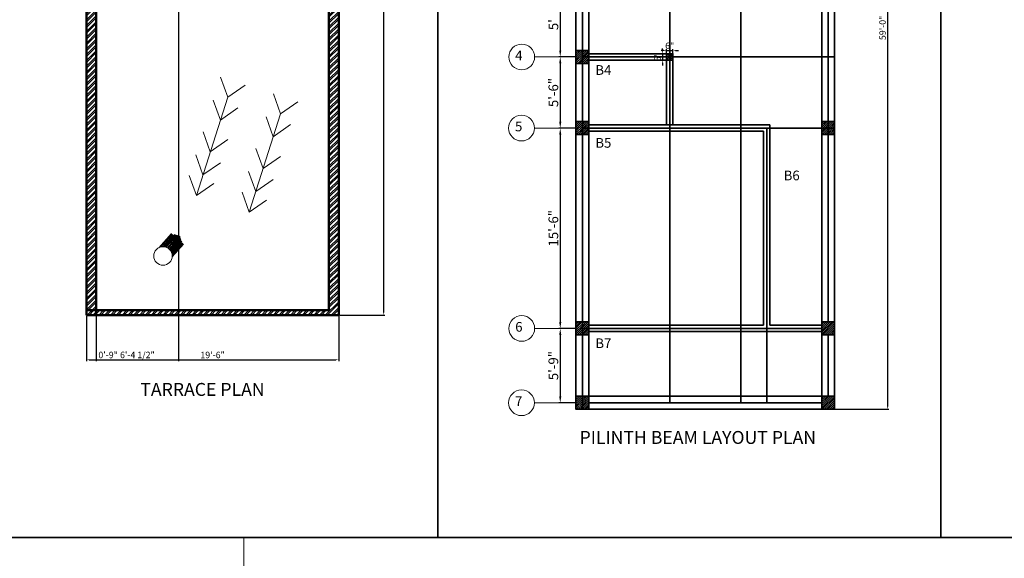
# Model space of a CAD drawing. Units: millimetres. Extents: x 20768 to 23556, y 50760 to 52704.
# Tile 30 of 36: x 21642 to 22556, y 51604 to 52104. Entities that reach past the tile are written whole.
import ezdxf

# ---------------------------------------------------------------- set-up
doc = ezdxf.new("R2010")
doc.units = ezdxf.units.MM
for name, color, linetype, lineweight in [('A-ANNO-SCHD', 7, 'Continuous', 18), ('A-ANNO-TEXT', 7, 'Continuous', 18), ('A-ANNO-TTLB', 7, 'Continuous', 35), ('A-ROOF', 30, 'Continuous', 18), ('A-WALL', 7, 'Continuous', 50), ('A-WALL-PATT', 8, 'Continuous', 13), ('S-ANNO-DIMS', 2, 'Continuous', 18), ('S-ANNO-TEXT', 6, 'Continuous', 18), ('S-BEAM', 3, 'Continuous', 35), ('S-COLS', 20, 'Continuous', 35), ('S-COLS-PATT', 8, 'Continuous', 13), ('S-GRID', 1, 'Continuous', 18)]:
    doc.layers.add(name, color=color, linetype=linetype, lineweight=lineweight)
doc.styles.get("Standard").update_dxf_attribs({"font": 'arial.ttf'})
doc.dimstyles.new('ISO-25', dxfattribs={"dimtxt": 6, "dimasz": 2.5, "dimexe": 1.25, "dimexo": 0.625, "dimtad": 1, "dimdec": 0, "dimlunit": 3, "dimtxsty": 'Standard', "dimcen": 2.5, "dimadec": 0, "dimazin": 0, "dimtfac": 1, "dimtdec": 0, "dimtmove": 0, "dimatfit": 3, "dimfxl": 1, "dimarcsym": 0})
pattern_1 = [(45, (102.9326, 0), (-0.898025612, 0.898025612), [])]

# ---------------------------------------------------------------- blocks, each defined once
blk = doc.blocks.new('*D37')
at = {"layer": 'Defpoints', "color": 0, "transparency": 16777216}
for p in [(22158.2, 52129.51), (22143.63, 52069.51), (22158.2, 52069.51)]:
    blk.add_point(p, dxfattribs=at)
at = {"layer": 'S-ANNO-DIMS', "color": 0, "lineweight": -2, "transparency": 16777216}
for p, q in [((22157.58, 52129.51), (22142.38, 52129.51)), ((22143.63, 52123.51), (22143.63, 52075.51)), ((22157.58, 52069.51), (22142.38, 52069.51))]:
    blk.add_line(p, q, dxfattribs=at)
at = {"layer": 'S-ANNO-DIMS', "color": 0, "transparency": 16777216}
for points in [[(22142.63, 52123.51), (22144.63, 52123.51), (22143.63, 52129.51)], [(22142.63, 52075.51), (22144.63, 52075.51), (22143.63, 52069.51)]]:
    blk.add_solid(points, dxfattribs=at)
at = {"layer": 'S-ANNO-DIMS', "color": 0, "transparency": 16777216, "insert": (22138.43, 52099.51), "char_height": 9, "attachment_point": 5, "rotation": 90}
blk.add_mtext("5'", dxfattribs=at)
blk = doc.blocks.new('*D38')
at = {"layer": 'Defpoints', "color": 0, "transparency": 16777216}
for p in [(22158.2, 52069.51), (22143.63, 52003.51), (22158.2, 52003.51)]:
    blk.add_point(p, dxfattribs=at)
at = {"layer": 'S-ANNO-DIMS', "color": 0, "lineweight": -2, "transparency": 16777216}
for p, q in [((22157.58, 52069.51), (22142.38, 52069.51)), ((22143.63, 52063.51), (22143.63, 52009.51)), ((22157.58, 52003.51), (22142.38, 52003.51))]:
    blk.add_line(p, q, dxfattribs=at)
at = {"layer": 'S-ANNO-DIMS', "color": 0, "transparency": 16777216}
for points in [[(22142.63, 52063.51), (22144.63, 52063.51), (22143.63, 52069.51)], [(22142.63, 52009.51), (22144.63, 52009.51), (22143.63, 52003.51)]]:
    blk.add_solid(points, dxfattribs=at)
at = {"layer": 'S-ANNO-DIMS', "color": 0, "transparency": 16777216, "insert": (22138.41, 52036.51), "char_height": 9, "attachment_point": 5, "rotation": 90}
blk.add_mtext('5\'-6"', dxfattribs=at)
blk = doc.blocks.new('*D39')
at = {"layer": 'Defpoints', "color": 0, "transparency": 16777216}
for p in [(22158.2, 52003.51), (22143.63, 51817.51), (22158.2, 51817.51)]:
    blk.add_point(p, dxfattribs=at)
at = {"layer": 'S-ANNO-DIMS', "color": 0, "lineweight": -2, "transparency": 16777216}
for p, q in [((22157.58, 52003.51), (22142.38, 52003.51)), ((22143.63, 51997.51), (22143.63, 51823.51)), ((22157.58, 51817.51), (22142.38, 51817.51))]:
    blk.add_line(p, q, dxfattribs=at)
at = {"layer": 'S-ANNO-DIMS', "color": 0, "transparency": 16777216}
for points in [[(22142.63, 51997.51), (22144.63, 51997.51), (22143.63, 52003.51)], [(22142.63, 51823.51), (22144.63, 51823.51), (22143.63, 51817.51)]]:
    blk.add_solid(points, dxfattribs=at)
at = {"layer": 'S-ANNO-DIMS', "color": 0, "transparency": 16777216, "insert": (22138.41, 51910.51), "char_height": 9, "attachment_point": 5, "rotation": 90}
blk.add_mtext('15\'-6"', dxfattribs=at)
blk = doc.blocks.new('*D40')
at = {"layer": 'Defpoints', "color": 0, "transparency": 16777216}
for p in [(22158.2, 51817.51), (22143.63, 51748.51), (22158.2, 51748.51)]:
    blk.add_point(p, dxfattribs=at)
at = {"layer": 'S-ANNO-DIMS', "color": 0, "lineweight": -2, "transparency": 16777216}
for p, q in [((22157.58, 51817.51), (22142.38, 51817.51)), ((22143.63, 51811.51), (22143.63, 51754.51)), ((22157.58, 51748.51), (22142.38, 51748.51))]:
    blk.add_line(p, q, dxfattribs=at)
at = {"layer": 'S-ANNO-DIMS', "color": 0, "transparency": 16777216}
for points in [[(22142.63, 51811.51), (22144.63, 51811.51), (22143.63, 51817.51)], [(22142.63, 51754.51), (22144.63, 51754.51), (22143.63, 51748.51)]]:
    blk.add_solid(points, dxfattribs=at)
at = {"layer": 'S-ANNO-DIMS', "color": 0, "transparency": 16777216, "insert": (22138.41, 51783.01), "char_height": 9, "attachment_point": 5, "rotation": 90}
blk.add_mtext('5\'-9"', dxfattribs=at)
blk = doc.blocks.new('*D43')
at = {"layer": 'Defpoints', "color": 0, "transparency": 16777216}
for p in [(22242.2, 52072.51), (22248.2, 52075.41), (22248.2, 52072.51)]:
    blk.add_point(p, dxfattribs=at)
at = {"layer": 'S-ANNO-DIMS', "color": 0, "lineweight": -2, "transparency": 16777216}
for p, q in [((22239.7, 52075.41), (22237.2, 52075.41)), ((22242.2, 52073.13), (22242.2, 52076.66)), ((22242.2, 52075.41), (22248.2, 52075.41)), ((22248.2, 52073.13), (22248.2, 52076.66)), ((22250.7, 52075.41), (22253.2, 52075.41))]:
    blk.add_line(p, q, dxfattribs=at)
at = {"layer": 'S-ANNO-DIMS', "color": 0, "transparency": 16777216}
for points in [[(22239.7, 52075.83), (22239.7, 52075), (22242.2, 52075.41)], [(22250.7, 52075.83), (22250.7, 52075), (22248.2, 52075.41)]]:
    blk.add_solid(points, dxfattribs=at)
at = {"layer": 'S-ANNO-DIMS', "color": 0, "transparency": 16777216, "insert": (22245.2, 52079.1), "char_height": 6, "attachment_point": 5}
blk.add_mtext('6"', dxfattribs=at)
blk = doc.blocks.new('*D44')
at = {"layer": 'Defpoints', "color": 0, "transparency": 16777216}
for p in [(22242.2, 52072.51), (22238.36, 52066.51), (22242.2, 52066.51)]:
    blk.add_point(p, dxfattribs=at)
at = {"layer": 'S-ANNO-DIMS', "color": 0, "lineweight": -2, "transparency": 16777216}
for p, q in [((22238.36, 52075.01), (22238.36, 52077.51)), ((22241.58, 52072.51), (22237.11, 52072.51)), ((22238.36, 52072.51), (22238.36, 52066.51)), ((22241.58, 52066.51), (22237.11, 52066.51)), ((22238.36, 52064.01), (22238.36, 52061.51))]:
    blk.add_line(p, q, dxfattribs=at)
at = {"layer": 'S-ANNO-DIMS', "color": 0, "transparency": 16777216}
for points in [[(22237.95, 52075.01), (22238.78, 52075.01), (22238.36, 52072.51)], [(22237.95, 52064.01), (22238.78, 52064.01), (22238.36, 52066.51)]]:
    blk.add_solid(points, dxfattribs=at)
at = {"layer": 'S-ANNO-DIMS', "color": 0, "transparency": 16777216, "insert": (22234.68, 52069.51), "char_height": 6, "attachment_point": 5, "rotation": 90}
blk.add_mtext('6"', dxfattribs=at)
blk = doc.blocks.new('GRID-BUBBLE')
blk.add_line((47.87, 11.93), (23.87, 11.93))
blk.add_circle((11.93, 11.93), 11.93)
blk = doc.blocks.new('*D217')
at = {"layer": 'Defpoints', "color": 0, "transparency": 16777216}
for p in [(21704.07, 51829.9), (21938.07, 51829.9), (21938.07, 51788.4)]:
    blk.add_point(p, dxfattribs=at)
at = {"layer": 'S-ANNO-DIMS', "color": 0, "lineweight": -2, "transparency": 16777216}
for p, q in [((21704.07, 51829.27), (21704.07, 51787.15)), ((21938.07, 51829.27), (21938.07, 51787.15)), ((21706.57, 51788.4), (21935.57, 51788.4))]:
    blk.add_line(p, q, dxfattribs=at)
at = {"layer": 'S-ANNO-DIMS', "color": 0, "transparency": 16777216}
for points in [[(21706.57, 51788.81), (21706.57, 51787.98), (21704.07, 51788.4)], [(21935.57, 51788.81), (21935.57, 51787.98), (21938.07, 51788.4)]]:
    blk.add_solid(points, dxfattribs=at)
at = {"layer": 'S-ANNO-DIMS', "color": 0, "transparency": 16777216, "insert": (21821.07, 51792.09), "char_height": 6, "attachment_point": 5}
blk.add_mtext('19\'-6"', dxfattribs=at)
blk = doc.blocks.new('*D218')
at = {"layer": 'Defpoints', "color": 0, "transparency": 16777216}
for p in [(21938.07, 52522.9), (21938.07, 51829.9), (21979.57, 51829.9)]:
    blk.add_point(p, dxfattribs=at)
at = {"layer": 'S-ANNO-DIMS', "color": 0, "lineweight": -2, "transparency": 16777216}
for p, q in [((21938.69, 52522.9), (21980.82, 52522.9)), ((21979.57, 52520.4), (21979.57, 51832.4)), ((21938.69, 51829.9), (21980.82, 51829.9))]:
    blk.add_line(p, q, dxfattribs=at)
at = {"layer": 'S-ANNO-DIMS', "color": 0, "transparency": 16777216}
for points in [[(21979.15, 52520.4), (21979.98, 52520.4), (21979.57, 52522.9)], [(21979.15, 51832.4), (21979.98, 51832.4), (21979.57, 51829.9)]]:
    blk.add_solid(points, dxfattribs=at)
at = {"layer": 'S-ANNO-DIMS', "color": 0, "transparency": 16777216, "insert": (21975.88, 52176.4), "char_height": 6, "attachment_point": 5, "rotation": 90}
blk.add_mtext('57\'-9"', dxfattribs=at)
blk = doc.blocks.new('*D219')
at = {"layer": 'Defpoints', "color": 0, "transparency": 16777216}
for p in [(21704.07, 51829.9), (21713.07, 51829.9), (21713.07, 51788.4)]:
    blk.add_point(p, dxfattribs=at)
at = {"layer": 'S-ANNO-DIMS', "color": 0, "lineweight": -2, "transparency": 16777216}
for p, q in [((21704.07, 51829.27), (21704.07, 51787.15)), ((21713.07, 51829.27), (21713.07, 51787.15)), ((21706.57, 51788.4), (21710.57, 51788.4)), ((21713.07, 51788.4), (21732.77, 51788.4))]:
    blk.add_line(p, q, dxfattribs=at)
at = {"layer": 'S-ANNO-DIMS', "color": 0, "transparency": 16777216}
for points in [[(21706.57, 51788.81), (21706.57, 51787.98), (21704.07, 51788.4)], [(21710.57, 51788.81), (21710.57, 51787.98), (21713.07, 51788.4)]]:
    blk.add_solid(points, dxfattribs=at)
at = {"layer": 'S-ANNO-DIMS', "color": 0, "transparency": 16777216, "insert": (21724.17, 51792.09), "char_height": 6, "attachment_point": 5}
blk.add_mtext('0\'-9"', dxfattribs=at)
blk = doc.blocks.new('*D222')
at = {"layer": 'Defpoints', "color": 0, "transparency": 16777216}
for p in [(21713.07, 52144.9), (21789.57, 52144.9), (21789.57, 51788.4)]:
    blk.add_point(p, dxfattribs=at)
at = {"layer": 'S-ANNO-DIMS', "color": 0, "lineweight": -2, "transparency": 16777216}
for p, q in [((21713.07, 52144.27), (21713.07, 51787.15)), ((21789.57, 52144.27), (21789.57, 51787.15)), ((21715.57, 51788.4), (21787.07, 51788.4))]:
    blk.add_line(p, q, dxfattribs=at)
at = {"layer": 'S-ANNO-DIMS', "color": 0, "transparency": 16777216}
for points in [[(21715.57, 51788.81), (21715.57, 51787.98), (21713.07, 51788.4)], [(21787.07, 51788.81), (21787.07, 51787.98), (21789.57, 51788.4)]]:
    blk.add_solid(points, dxfattribs=at)
at = {"layer": 'S-ANNO-DIMS', "color": 0, "transparency": 16777216, "insert": (21751.32, 51792.12), "char_height": 6, "attachment_point": 5}
blk.add_mtext('6\'-4 1/2"', dxfattribs=at)
blk = doc.blocks.new('*D224')
at = {"layer": 'Defpoints', "color": 0, "transparency": 16777216}
for p in [(22398.2, 52450.51), (22398.2, 51742.51), (22447.14, 51742.51)]:
    blk.add_point(p, dxfattribs=at)
at = {"layer": 'S-ANNO-DIMS', "color": 0, "lineweight": -2, "transparency": 16777216}
for p, q in [((22398.83, 52450.51), (22448.39, 52450.51)), ((22447.14, 52448.01), (22447.14, 51745.01)), ((22398.83, 51742.51), (22448.39, 51742.51))]:
    blk.add_line(p, q, dxfattribs=at)
at = {"layer": 'S-ANNO-DIMS', "color": 0, "transparency": 16777216}
for points in [[(22446.72, 52448.01), (22447.56, 52448.01), (22447.14, 52450.51)], [(22446.72, 51745.01), (22447.56, 51745.01), (22447.14, 51742.51)]]:
    blk.add_solid(points, dxfattribs=at)
at = {"layer": 'S-ANNO-DIMS', "color": 0, "transparency": 16777216, "insert": (22443.45, 52096.51), "char_height": 6, "attachment_point": 5, "rotation": 90}
blk.add_mtext('59\'-0"', dxfattribs=at)

msp = doc.modelspace()

# ---------------------------------------------------------------- hatches: boundary and pattern name
at = {"layer": 'A-WALL-PATT'}
h = msp.add_hatch(dxfattribs=at)
h.set_pattern_fill('ANSI32', color=256, scale=0.4)
h.paths.add_polyline_path([(21713.07, 52513.9), (21929.07, 52513.9), (21929.07, 51834.4), (21713.07, 51834.4), (21713.07, 51829.9), (21938.07, 51829.9), (21938.07, 52522.9), (21704.07, 52522.9), (21704.07, 51834.4), (21713.07, 51834.4)])
h = msp.add_hatch(dxfattribs=at)
h.set_pattern_fill('ANSI32', color=256, scale=0.4)
h.paths.add_polyline_path([(21713.07, 51834.4), (21704.07, 51834.4), (21704.07, 51829.9), (21713.07, 51829.9)])
at = {"layer": 'S-COLS-PATT'}
h = msp.add_hatch(dxfattribs=at)
h.set_pattern_fill('ANSI31', color=256, scale=0.4)
h.set_pattern_definition(pattern_1)
h.paths.add_polyline_path([(22164.2, 52075.51), (22158.2, 52075.51), (22158.2, 52063.51), (22164.2, 52063.51)])
h = msp.add_hatch(dxfattribs=at)
h.set_pattern_fill('ANSI31', color=256, scale=0.4)
h.set_pattern_definition(pattern_1)
h.paths.add_polyline_path([(22170.2, 52075.51), (22164.2, 52075.51), (22164.2, 52069.51), (22170.2, 52069.51)])
h = msp.add_hatch(dxfattribs=at)
h.set_pattern_fill('ANSI31', color=256, scale=0.4)
h.set_pattern_definition(pattern_1)
h.paths.add_polyline_path([(22170.2, 52069.51), (22164.2, 52069.51), (22164.2, 52063.51), (22170.2, 52063.51)])
h = msp.add_hatch(dxfattribs=at)
h.set_pattern_fill('ANSI31', color=256, scale=0.4)
h.set_pattern_definition(pattern_1)
h.paths.add_polyline_path([(22245.2, 52072.51), (22242.2, 52072.51), (22242.2, 52069.51), (22245.2, 52069.51)])
h = msp.add_hatch(dxfattribs=at)
h.set_pattern_fill('ANSI31', color=256, scale=0.4)
h.set_pattern_definition(pattern_1)
h.paths.add_polyline_path([(22245.2, 52069.51), (22242.2, 52069.51), (22242.2, 52066.51), (22245.2, 52066.51)])
h = msp.add_hatch(dxfattribs=at)
h.set_pattern_fill('ANSI31', color=256, scale=0.4)
h.set_pattern_definition(pattern_1)
h.paths.add_polyline_path([(22248.2, 52072.51), (22245.2, 52072.51), (22245.2, 52069.51), (22248.2, 52069.51)], flags=17)
h = msp.add_hatch(dxfattribs=at)
h.set_pattern_fill('ANSI31', color=256, scale=0.4)
h.set_pattern_definition(pattern_1)
h.paths.add_polyline_path([(22248.2, 52069.51), (22245.2, 52069.51), (22245.2, 52066.51), (22248.2, 52066.51)])
h = msp.add_hatch(dxfattribs=at)
h.set_pattern_fill('ANSI31', color=256, scale=0.4)
h.set_pattern_definition(pattern_1)
h.paths.add_polyline_path([(22164.2, 52009.51), (22158.2, 52009.51), (22158.2, 51997.51), (22164.2, 51997.51)])
h = msp.add_hatch(dxfattribs=at)
h.set_pattern_fill('ANSI31', color=256, scale=0.4)
h.set_pattern_definition(pattern_1)
h.paths.add_polyline_path([(22170.2, 52009.51), (22164.2, 52009.51), (22164.2, 52003.51), (22170.2, 52003.51)])
h = msp.add_hatch(dxfattribs=at)
h.set_pattern_fill('ANSI31', color=256, scale=0.4)
h.set_pattern_definition(pattern_1)
h.paths.add_polyline_path([(22392.2, 52009.51), (22386.2, 52009.51), (22386.2, 52003.51), (22392.2, 52003.51)])
h = msp.add_hatch(dxfattribs=at)
h.set_pattern_fill('ANSI31', color=256, scale=0.4)
h.set_pattern_definition(pattern_1)
h.paths.add_polyline_path([(22398.2, 52009.51), (22392.2, 52009.51), (22392.2, 52003.51), (22398.2, 52003.51)])
h = msp.add_hatch(dxfattribs=at)
h.set_pattern_fill('ANSI31', color=256, scale=0.4)
h.set_pattern_definition(pattern_1)
h.paths.add_polyline_path([(22170.2, 52003.51), (22164.2, 52003.51), (22164.2, 51997.51), (22170.2, 51997.51)])
h = msp.add_hatch(dxfattribs=at)
h.set_pattern_fill('ANSI31', color=256, scale=0.4)
h.set_pattern_definition(pattern_1)
h.paths.add_polyline_path([(22392.2, 52003.51), (22386.2, 52003.51), (22386.2, 51997.51), (22392.2, 51997.51)])
h = msp.add_hatch(dxfattribs=at)
h.set_pattern_fill('ANSI31', color=256, scale=0.4)
h.set_pattern_definition(pattern_1)
h.paths.add_polyline_path([(22398.2, 52003.51), (22392.2, 52003.51), (22392.2, 51997.51), (22398.2, 51997.51)])
h = msp.add_hatch(dxfattribs=at)
h.set_pattern_fill('ANSI31', color=256, scale=0.4)
h.set_pattern_definition(pattern_1)
h.paths.add_polyline_path([(22164.2, 51823.51), (22158.2, 51823.51), (22158.2, 51811.51), (22164.2, 51811.51)])
h = msp.add_hatch(dxfattribs=at)
h.set_pattern_fill('ANSI31', color=256, scale=0.4)
h.set_pattern_definition(pattern_1)
h.paths.add_polyline_path([(22170.2, 51823.51), (22164.2, 51823.51), (22164.2, 51817.51), (22170.2, 51817.51)])
h = msp.add_hatch(dxfattribs=at)
h.set_pattern_fill('ANSI31', color=256, scale=0.4)
h.set_pattern_definition(pattern_1)
h.paths.add_polyline_path([(22398.2, 51823.51), (22386.2, 51823.51), (22386.2, 51811.51), (22398.2, 51811.51)])
h = msp.add_hatch(dxfattribs=at)
h.set_pattern_fill('ANSI31', color=256, scale=0.4)
h.set_pattern_definition(pattern_1)
h.paths.add_polyline_path([(22170.2, 51817.51), (22164.2, 51817.51), (22164.2, 51811.51), (22170.2, 51811.51)])
h = msp.add_hatch(dxfattribs=at)
h.set_pattern_fill('ANSI31', color=256, scale=0.4)
h.set_pattern_definition(pattern_1)
h.paths.add_polyline_path([(22164.2, 51754.51), (22158.2, 51754.51), (22158.2, 51742.51), (22164.2, 51742.51)])
h = msp.add_hatch(dxfattribs=at)
h.set_pattern_fill('ANSI31', color=256, scale=0.4)
h.set_pattern_definition(pattern_1)
h.paths.add_polyline_path([(22170.2, 51754.51), (22164.2, 51754.51), (22164.2, 51742.51), (22170.2, 51742.51)])
h = msp.add_hatch(dxfattribs=at)
h.set_pattern_fill('ANSI31', color=256, scale=0.4)
h.set_pattern_definition(pattern_1)
h.paths.add_polyline_path([(22398.2, 51754.51), (22386.2, 51754.51), (22386.2, 51742.51), (22398.2, 51742.51)])

# ---------------------------------------------------------------- linework, layer by layer
at = {"layer": 'A-ANNO-SCHD'}
msp.add_line((21849.94, 51623.53), (21849.94, 50975.78), dxfattribs=at)
at = {"layer": 'A-ANNO-TTLB'}
for p, q in [((22029.91, 52703.98), (22029.91, 51623.53)), ((22496.64, 52703.98), (22496.64, 51623.53))]:
    msp.add_line(p, q, dxfattribs=at)
msp.add_lwpolyline([(20768.14, 52703.98), (23555.8, 52703.98), (23555.8, 51623.53), (20768.14, 51623.53)], close=True, dxfattribs=at)
at = {"layer": 'A-ROOF'}
for p, q in [((21835.15, 52032.28), (21806.04, 51940.94)), ((21884.18, 52016.77), (21855.07, 51925.44)), ((21771.15, 51892.42), (21782.92, 51905.77)), ((21773.12, 51893.14), (21783.67, 51905.11)), ((21774.65, 51893.36), (21784.42, 51904.44)), ((21775.95, 51893.32), (21785.91, 51904.62)), ((21777.11, 51893.13), (21786.93, 51904.27)), ((21778.16, 51892.8), (21788.15, 51904.14)), ((21779.11, 51892.37), (21789.35, 51903.99)), ((21780.01, 51891.88), (21790.29, 51903.54)), ((21780.76, 51891.22), (21791.02, 51902.86)), ((21781.51, 51890.56), (21791.22, 51901.57)), ((21782.11, 51889.72), (21791.63, 51900.52)), ((21782.66, 51888.83), (21791.82, 51899.23)), ((21783.11, 51887.84), (21792.49, 51898.47)), ((21783.45, 51886.71), (21792.67, 51897.17)), ((21783.63, 51883.88), (21794.17, 51895.85)), ((21783.65, 51885.42), (21793.42, 51896.51))]:
    msp.add_line(p, q, dxfattribs=at)
for points in [[(21828.49, 52050.74), (21835.15, 52032.28), (21851.27, 52043.48)], [(21877.51, 52035.24), (21884.18, 52016.77), (21900.3, 52027.98)], [(21821.7, 52029.47), (21828.37, 52011), (21844.49, 52022.2)], [(21870.73, 52013.96), (21877.4, 51995.5), (21893.52, 52006.7)], [(21812.33, 52000.04), (21818.99, 51981.57), (21835.11, 51992.78)], [(21805.5, 51978.63), (21812.17, 51960.16), (21828.29, 51971.36)], [(21861.35, 51984.54), (21868.02, 51966.07), (21884.14, 51977.27)], [(21799.38, 51959.41), (21806.04, 51940.94), (21822.16, 51952.15)], [(21854.53, 51963.12), (21861.19, 51944.66), (21877.31, 51955.86)], [(21848.4, 51943.91), (21855.07, 51925.44), (21871.19, 51936.65)]]:
    msp.add_lwpolyline(points, dxfattribs=at)
msp.add_circle((21775.08, 51884.78), 8.59, dxfattribs=at)
at = {"layer": 'A-WALL'}
for p, q in [((21704.07, 52522.9), (21704.07, 51829.9)), ((21938.07, 52522.9), (21938.07, 51829.9)), ((21713.07, 52513.9), (21713.07, 51829.9)), ((21929.07, 52513.9), (21929.07, 51834.4)), ((21704.07, 51834.4), (21929.07, 51834.4)), ((21704.07, 51829.9), (21938.07, 51829.9))]:
    msp.add_line(p, q, dxfattribs=at)
at = {"layer": 'S-BEAM'}
for p, q in [((22158.2, 52450.51), (22158.2, 51742.51)), ((22164.2, 52444.51), (22164.2, 51742.51)), ((22170.2, 52450.51), (22170.2, 51742.51)), ((22245.2, 52444.51), (22245.2, 51748.51)), ((22311.2, 52444.51), (22311.2, 51748.51)), ((22386.2, 52450.51), (22386.2, 51742.51)), ((22398.2, 52450.51), (22398.2, 51742.51)), ((22392.2, 52123.51), (22392.2, 51823.51)), ((22164.2, 52069.51), (22398.2, 52069.51)), ((22170.2, 52072.51), (22248.2, 52072.51)), ((22242.2, 52072.51), (22242.2, 52006.51)), ((22248.2, 52072.51), (22248.2, 52006.51)), ((22170.2, 52066.51), (22248.2, 52066.51)), ((22170.2, 52006.51), (22338.2, 52006.51)), ((22338.2, 52006.51), (22338.2, 51820.51)), ((22164.2, 52003.51), (22398.2, 52003.51)), ((22170.2, 52000.51), (22332.2, 52000.51)), ((22332.2, 52000.51), (22332.2, 51820.51)), ((22335.2, 52003.51), (22335.2, 51748.51)), ((22164.2, 51817.51), (22386.2, 51817.51)), ((22170.2, 51820.51), (22332.2, 51820.51)), ((22170.2, 51814.51), (22386.2, 51814.51)), ((22338.2, 51820.51), (22386.2, 51820.51)), ((22392.2, 51811.51), (22392.2, 51754.51)), ((22170.2, 51754.51), (22398.2, 51754.51)), ((22158.2, 51742.51), (22398.2, 51742.51)), ((22170.2, 51748.51), (22386.2, 51748.51))]:
    msp.add_line(p, q, dxfattribs=at)
at = {"layer": 'S-COLS'}
for points in [[(22170.2, 52075.51), (22158.2, 52075.51), (22158.2, 52063.51), (22170.2, 52063.51)], [(22242.2, 52072.51), (22248.2, 52072.51), (22248.2, 52066.51), (22242.2, 52066.51)], [(22170.2, 52009.51), (22158.2, 52009.51), (22158.2, 51997.51), (22170.2, 51997.51)], [(22386.2, 52009.51), (22398.2, 52009.51), (22398.2, 51997.51), (22386.2, 51997.51)], [(22170.2, 51823.51), (22158.2, 51823.51), (22158.2, 51811.51), (22170.2, 51811.51)], [(22386.2, 51823.51), (22398.2, 51823.51), (22398.2, 51811.51), (22386.2, 51811.51)], [(22170.2, 51754.51), (22158.2, 51754.51), (22158.2, 51742.51), (22170.2, 51742.51)], [(22386.2, 51754.51), (22398.2, 51754.51), (22398.2, 51742.51), (22386.2, 51742.51)]]:
    msp.add_lwpolyline(points, close=True, dxfattribs=at)

# ---------------------------------------------------------------- block references
at = {"layer": 'S-GRID'}
for p in [(22095.97, 52057.57), (22095.76, 51991.57), (22095.97, 51805.57), (22095.76, 51736.57)]:
    msp.add_blockref('GRID-BUBBLE', p, dxfattribs=at)

# ---------------------------------------------------------------- texts
at = {"layer": 'A-ANNO-TEXT', "insert": (21754.04, 51766.88), "char_height": 12, "attachment_point": 1}
msp.add_mtext_dynamic_manual_height_columns('TARRACE PLAN', width=206.7681, gutter_width=12.5, heights=[0], dxfattribs=at)
at = {"layer": 'S-ANNO-TEXT', "attachment_point": 1}
for s, width, insert, char_height in [('  4', 27.5349, (22096.36, 52075.48), 9), ('B4', 18.885, (22176.18, 52061.91), 9), ('  5', 27.5349, (22096.15, 52009.48), 9), ('B5', 18.885, (22176.18, 51994.28), 9), ('B6', 18.885, (22350.91, 51964.01), 9), ('  6', 27.5349, (22096.36, 51823.48), 9), ('B7', 18.885, (22176.18, 51808.24), 9), ('  7', 27.5349, (22096.15, 51754.48), 9), ('PILINTH BEAM LAYOUT PLAN', 241.5904, (22161.55, 51722.3), 12)]:
    msp.add_mtext_dynamic_manual_height_columns(s, width=width, gutter_width=12.5, heights=[0], dxfattribs=dict(at, insert=insert, char_height=char_height))

# ---------------------------------------------------------------- dimensions: what is measured, and where the dimension line sits
at = {"layer": 'S-ANNO-DIMS'}
for base, p1, p2, override, picture, middle in [((21979.57, 51829.9), (21938.07, 52522.9), (21938.07, 51829.9), {"dimdec": 1, "dimlfac": 1, "dimrnd": 0, "dimzin": 1, "dimdsep": 46, "dimlunit": 4, "dimfrac": 2}, '*D218', (21975.88, 52176.4)), ((22447.14, 51742.51), (22398.2, 52450.51), (22398.2, 51742.51), {"dimdec": 1, "dimlfac": 1, "dimrnd": 0, "dimzin": 1, "dimdsep": 46, "dimlunit": 4, "dimfrac": 2}, '*D224', (22443.45, 52096.51)), ((22143.63, 52069.51), (22158.2, 52129.51), (22158.2, 52069.51), {"dimtxt": 9, "dimasz": 6, "dimclrd": 0, "dimclre": 0, "dimclrt": 0}, '*D37', (22138.43, 52099.51)), ((22143.63, 52003.51), (22158.2, 52069.51), (22158.2, 52003.51), {"dimtxt": 9, "dimasz": 6, "dimclrd": 0, "dimclre": 0, "dimclrt": 0}, '*D38', (22138.41, 52036.51)), ((22143.63, 51817.51), (22158.2, 52003.51), (22158.2, 51817.51), {"dimtxt": 9, "dimasz": 6, "dimclrd": 0, "dimclre": 0, "dimclrt": 0}, '*D39', (22138.41, 51910.51)), ((22143.63, 51748.51), (22158.2, 51817.51), (22158.2, 51748.51), {"dimtxt": 9, "dimasz": 6, "dimclrd": 0, "dimclre": 0, "dimclrt": 0}, '*D40', (22138.41, 51783.01))]:
    dim = msp.add_linear_dim(base=base, p1=p1, p2=p2, angle=90, dimstyle='ISO-25', override=override, dxfattribs=at)
    dim.commit()
    dim.dimension.update_dxf_attribs({"geometry": picture, "text_midpoint": middle})
for base, p1, p2, picture, middle in [((21789.57, 51788.4), (21713.07, 52144.9), (21789.57, 52144.9), '*D222', (21751.32, 51792.12)), ((21938.07, 51788.4), (21704.07, 51829.9), (21938.07, 51829.9), '*D217', (21821.07, 51792.09)), ((21713.07, 51788.4), (21704.07, 51829.9), (21713.07, 51829.9), '*D219', (21724.17, 51792.09))]:
    dim = msp.add_linear_dim(base=base, p1=p1, p2=p2, dimstyle='ISO-25', override={"dimdec": 1, "dimlfac": 1, "dimrnd": 0, "dimzin": 1, "dimdsep": 46, "dimlunit": 4, "dimfrac": 2}, dxfattribs=at)
    dim.commit()
    dim.dimension.update_dxf_attribs({"geometry": picture, "text_midpoint": middle})
dim = msp.add_linear_dim(base=(22238.36, 52066.51), p1=(22242.2, 52072.51), p2=(22242.2, 52066.51), angle=90, dimstyle='ISO-25', override={"dimclrd": 0, "dimclre": 0, "dimclrt": 0}, dxfattribs=at)
dim.commit()
dim.dimension.update_dxf_attribs({"geometry": '*D44', "text_midpoint": (22238.36, 52069.51), "dimtype": 160})
dim = msp.add_linear_dim(base=(22248.2, 52075.41), p1=(22242.2, 52072.51), p2=(22248.2, 52072.51), dimstyle='ISO-25', override={"dimclrd": 0, "dimclre": 0, "dimclrt": 0}, dxfattribs=at)
dim.commit()
dim.dimension.update_dxf_attribs({"geometry": '*D43', "text_midpoint": (22245.2, 52075.41), "dimtype": 160})

doc.saveas('drawing.dxf')
